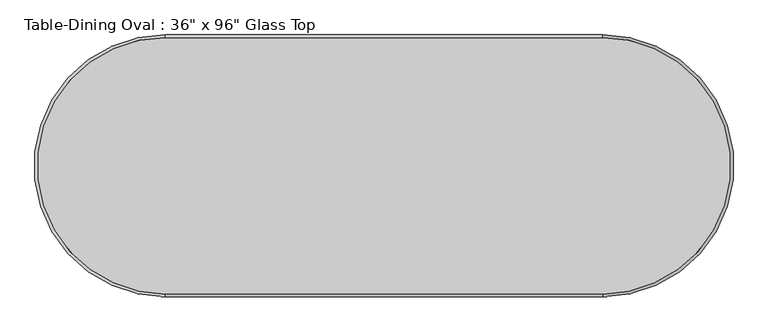
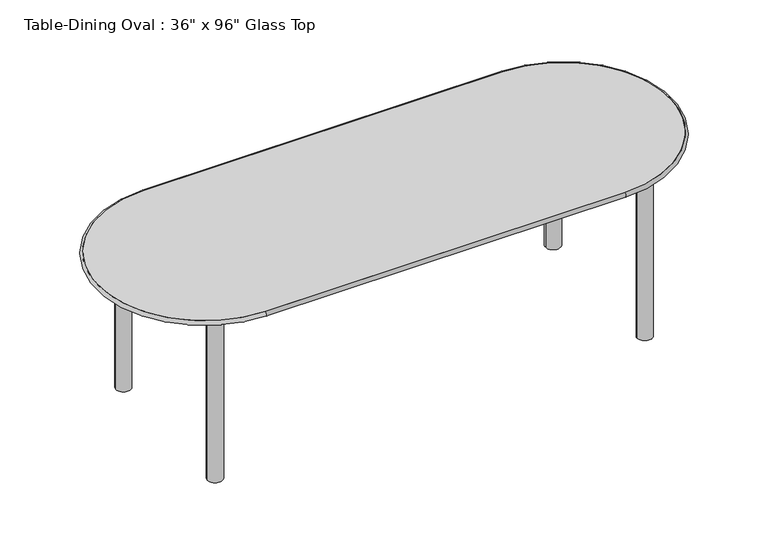
"""IFC4 building model written with IfcOpenShell, lengths in millimetres: furniture geometry."""

from ifc_helpers import new_model, si_unit, point, frame, frame_2d, origin, origin_with_axes, place, context, project, spatial, polyline, circle_curve, ellipse_curve, trimmed, segment, composite_curve, outline, extrude, source, transform, mapped, element, save
from ifc_brep_helpers import plane_surface, cylinder_surface, revolved_surface, advanced_brep


def furniture_e05f6f82(model_context):
    return source(origin(), model_context, "Body", "SolidModel", [
        advanced_brep(
        [(-1163.8196721, -805.7733607, 762.0), (-1163.8196721, -805.7733607, 742.95), (360.1803279, -805.7733607, 742.95), (360.1803279, -805.7733607, 762.0), (360.1803279, 89.5766393, 762.0), (360.1803279, 89.5766393, 742.95), (-1163.8196721, 89.5766393, 742.95), (-1163.8196721, 89.5766393, 762.0)],
        [
            (0, 1, circle_curve(frame((-1163.8196721, -805.7733607, 752.475), z_axis=(1.0, 0.0, 0.0), x_axis=(0.0, 1.0, 0.0)), 9.525)),
            (1, 2),
            (2, 3, circle_curve(frame((360.1803279, -805.7733607, 752.475), z_axis=(-1.0, 0.0, 0.0), x_axis=(0.0, 1.0, 0.0)), 9.525)),
            (3, 0),
            (1, 0),
            (3, 2),
            (4, 3, circle_curve(frame((360.1803279, -358.0983607, 762.0), z_axis=(0.0, 0.0, -1.0), x_axis=(0.0, -1.0, 0.0)), 447.675)),
            (2, 5, circle_curve(frame((360.1803279, -358.0983607, 742.95), z_axis=(0.0, 0.0, 1.0), x_axis=(0.0, -1.0, 0.0)), 447.675)),
            (5, 4, circle_curve(frame((360.1803279, 89.5766393, 752.475), z_axis=(1.0, 0.0, 0.0), x_axis=(0.0, -1.0, 0.0)), 9.525)),
            (4, 5),
            (5, 6),
            (6, 7, circle_curve(frame((-1163.8196721, 89.5766393, 752.475), z_axis=(1.0, 0.0, 0.0), x_axis=(0.0, -1.0, 0.0)), 9.525)),
            (7, 4),
            (7, 6),
            (0, 7, circle_curve(frame((-1163.8196721, -358.0983607, 762.0), z_axis=(0.0, 0.0, -1.0), x_axis=(0.0, 1.0, 0.0)), 447.675)),
            (6, 1, circle_curve(frame((-1163.8196721, -358.0983607, 742.95), z_axis=(0.0, 0.0, 1.0), x_axis=(0.0, 1.0, 0.0)), 447.675)),
        ],
        [
            cylinder_surface(frame((-1163.8196721, -805.7733607, 752.475), z_axis=(-1.0, 0.0, 0.0), x_axis=(0.0, 1.0, 0.0)), 9.525),
            plane_surface(frame((-1163.8196721, -805.7733607, 762.0), z_axis=(0.0, 1.0, 0.0), x_axis=(1.0, 0.0, 0.0))),
            revolved_surface(trimmed(ellipse_curve(frame((360.1803279, -805.7733607, 752.475), z_axis=(-1.0, 0.0, 0.0), x_axis=(0.0, 1.0, 0.0)), 9.525, 9.525), [point((360.1803279, -805.7733607, 742.95))], [point((360.1803279, -805.7733607, 762.0))], True, "CARTESIAN"), (360.1803279, -358.0983607, 0.0), (0.0, 0.0, 1.0)),
            revolved_surface(polyline([(360.1803279, -805.7733607, 762.0), (360.1803279, -805.7733607, 742.95)]), (360.1803279, -358.0983607, 0.0), (0.0, 0.0, 1.0)),
            cylinder_surface(frame((360.1803279, 89.5766393, 752.475), z_axis=(1.0, 0.0, 0.0), x_axis=(0.0, -1.0, 0.0)), 9.525),
            plane_surface(frame((360.1803279, 89.5766393, 762.0), z_axis=(0.0, -1.0, 0.0), x_axis=(-1.0, 0.0, 0.0))),
            revolved_surface(trimmed(ellipse_curve(frame((-1163.8196721, 89.5766393, 752.475), z_axis=(1.0, 0.0, 0.0), x_axis=(0.0, -1.0, 0.0)), 9.525, 9.525), [point((-1163.8196721, 89.5766393, 742.95))], [point((-1163.8196721, 89.5766393, 762.0))], True, "CARTESIAN"), (-1163.8196721, -358.0983607, 0.0), (0.0, 0.0, 1.0)),
            revolved_surface(polyline([(-1163.8196721, 89.57663930000001, 762.0), (-1163.8196721, 89.57663930000001, 742.95)]), (-1163.8196721, -358.0983607, 0.0), (0.0, 0.0, 1.0)),
        ],
        [
            (0, [[1, 2, 3, 4]]),
            (1, [[5, -4, 6, -2]]),
            (2, [[7, -3, 8, 9]]),
            (3, [[-8, -6, -7, 10]]),
            (4, [[-9, 11, 12, 13]]),
            (5, [[-10, -13, 14, -11]]),
            (6, [[15, -12, 16, -1]]),
            (7, [[-16, -14, -15, -5]]),
        ],
    ),
        extrude(outline(composite_curve([segment(trimmed(circle_curve(frame_2d((-1313.0446721, -21.5483607)), 31.75), [point((-1344.7946721, -21.5483607))], [point((-1281.2946721, -21.5483607))], False, "CARTESIAN"), True, "CONTINUOUS"), segment(trimmed(circle_curve(frame_2d((-1313.0446721, -21.5483607)), 31.75), [point((-1281.2946721, -21.5483607))], [point((-1344.7946721, -21.5483607))], False, "CARTESIAN"), True, "CONTINUOUS")], self_intersect=False)), origin_with_axes(), (0.0, 0.0, 1.0), 742.95),
        extrude(outline(composite_curve([segment(trimmed(circle_curve(frame_2d((-1313.0446721, -694.6483607)), 31.75), [point((-1344.7946721, -694.6483607))], [point((-1281.2946721, -694.6483607))], False, "CARTESIAN"), True, "CONTINUOUS"), segment(trimmed(circle_curve(frame_2d((-1313.0446721, -694.6483607)), 31.75), [point((-1281.2946721, -694.6483607))], [point((-1344.7946721, -694.6483607))], False, "CARTESIAN"), True, "CONTINUOUS")], self_intersect=False)), origin_with_axes(), (0.0, 0.0, 1.0), 742.95),
        extrude(outline(composite_curve([segment(trimmed(circle_curve(frame_2d((509.4053279, -21.5483607)), 31.75), [point((477.6553279, -21.5483607))], [point((541.1553279, -21.5483607))], False, "CARTESIAN"), True, "CONTINUOUS"), segment(trimmed(circle_curve(frame_2d((509.4053279, -21.5483607)), 31.75), [point((541.1553279, -21.5483607))], [point((477.6553279, -21.5483607))], False, "CARTESIAN"), True, "CONTINUOUS")], self_intersect=False)), origin_with_axes(), (0.0, 0.0, 1.0), 742.95),
        extrude(outline(composite_curve([segment(trimmed(circle_curve(frame_2d((509.4053279, -694.6483607)), 31.75), [point((477.6553279, -694.6483607))], [point((541.1553279, -694.6483607))], False, "CARTESIAN"), True, "CONTINUOUS"), segment(trimmed(circle_curve(frame_2d((509.4053279, -694.6483607)), 31.75), [point((541.1553279, -694.6483607))], [point((477.6553279, -694.6483607))], False, "CARTESIAN"), True, "CONTINUOUS")], self_intersect=False)), origin_with_axes(), (0.0, 0.0, 1.0), 742.95),
        extrude(outline(polyline([(528.4553279, -2.4983607), (528.4553279, -713.6983607), (-1332.0946721, -713.6983607), (-1332.0946721, -2.4983607), (528.4553279, -2.4983607)]), holes=[polyline([(509.4053279, -21.5483607), (-1313.0446721, -21.5483607), (-1313.0446721, -694.6483607), (509.4053279, -694.6483607), (509.4053279, -21.5483607)])]), frame((0.0, 0.0, 692.15), z_axis=(0.0, 0.0, 1.0), x_axis=(1.0, 0.0, 0.0)), (0.0, 0.0, 1.0), 50.8),
        extrude(outline(composite_curve([segment(polyline([(-1163.8196721, 89.5766393), (360.1803279, 89.5766393)]), True, "CONTINUOUS"), segment(trimmed(circle_curve(frame_2d((360.1803279, -358.0983607)), 447.675), [point((360.1803279, 89.5766393))], [point((807.8553279, -358.0983607))], False, "CARTESIAN"), True, "CONTINUOUS"), segment(trimmed(circle_curve(frame_2d((360.1803279, -358.0983607)), 447.675), [point((807.8553279, -358.0983607))], [point((360.1803279, -805.7733607))], False, "CARTESIAN"), True, "CONTINUOUS"), segment(polyline([(360.1803279, -805.7733607), (-1163.8196721, -805.7733607)]), True, "CONTINUOUS"), segment(trimmed(circle_curve(frame_2d((-1163.8196721, -358.0983607)), 447.675), [point((-1163.8196721, -805.7733607))], [point((-1611.4946721, -358.0983607))], False, "CARTESIAN"), True, "CONTINUOUS"), segment(trimmed(circle_curve(frame_2d((-1163.8196721, -358.0983607)), 447.675), [point((-1611.4946721, -358.0983607))], [point((-1163.8196721, 89.5766393))], False, "CARTESIAN"), True, "CONTINUOUS")], self_intersect=False)), frame((0.0, 0.0, 742.95), z_axis=(0.0, 0.0, 1.0), x_axis=(1.0, 0.0, 0.0)), (0.0, 0.0, 1.0), 19.05),
    ])


if __name__ == "__main__":
    model = new_model("IFC4")
    model_context = context("Model", 3, world=origin())
    ifc_project = project(units=[si_unit("LENGTHUNIT", "METRE", prefix="MILLI")], contexts=[model_context])
    site = spatial("IfcSite", under=ifc_project)
    building = spatial("IfcBuilding", under=site)
    placement = place(None, origin())
    furniture_shape = furniture_e05f6f82(model_context)
    element("IfcFurniture", 1, ObjectType="Table-Dining Oval : 36\" x 96\" Glass Top", at=placement, inside=building, context=model_context, shape_type="MappedRepresentation", body=[
        mapped(furniture_shape, transform((0.0, 0.0, 0.0), x_axis=(1.0, 0.0, 0.0), y_axis=(0.0, 1.0, 0.0), z_axis=(0.0, 0.0, 1.0))),
    ])
    save(model, "model.ifc")

# Revit data of these elements
# Type "Table-Dining Oval : 36\" x 96\" Glass Top"
#   Assembly Code = "E2020200"
#   Length = 8' - 0"
#   Width = 3' - 0"
#   Base Material = Steel, Chrome Plated
#   Top Material = Glass - Clear, Grey
#   Default Elevation = 0
#   Description = (empty or 0)
# Element 1 (IfcFurniture, "Table-Dining Oval : 36\" x 96\" Glass Top")
#   Materials on its faces: "Steel, Chrome Plated", "Glass - Clear, Grey"
# Materials
#   "Steel, Chrome Plated": class "Metal", colour RGB 17 17 17, transparency 0, Description = "Chromiuim plated steel", Cost = 0
#   "Glass - Clear, Grey": class "Glass", colour RGB 252 255 255, transparency 0.64
